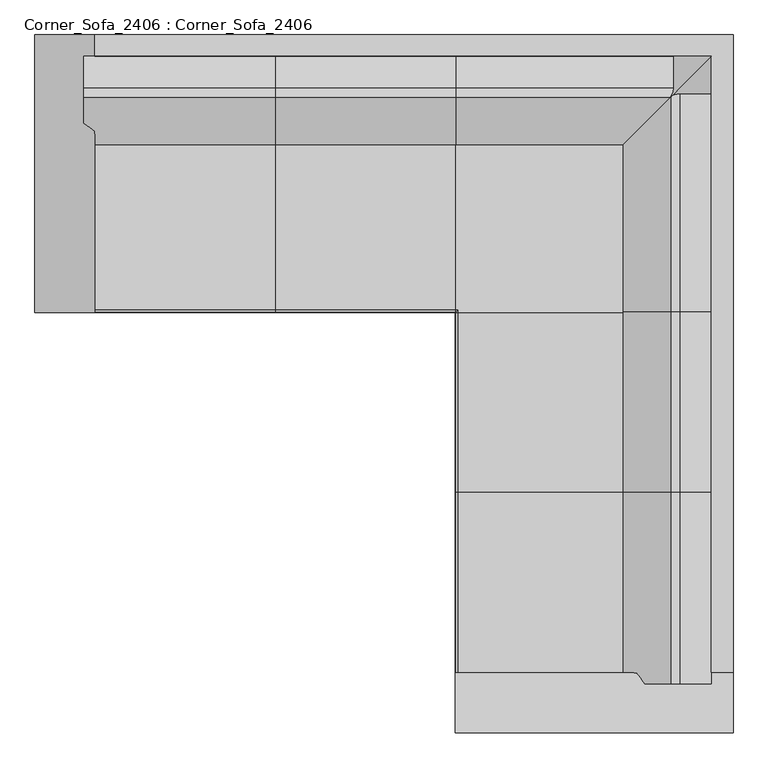
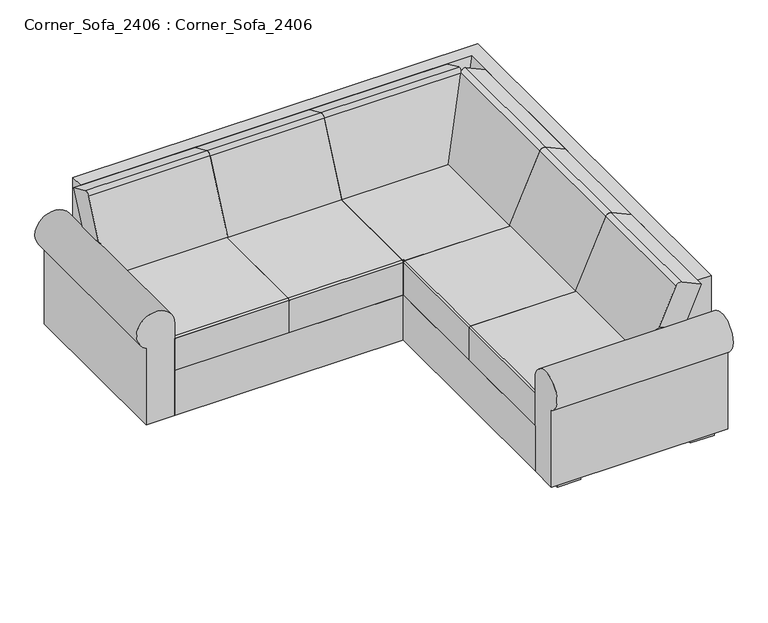
"""IFC4 building model written with IfcOpenShell, lengths in millimetres: furniture geometry, Corner_Sofa_2406 : Corner_Sofa_2406."""

from ifc_helpers import new_model, si_unit, point, frame, frame_2d, origin, origin_with_axes, place, context, project, spatial, polyline, circle_curve, ellipse_curve, trimmed, segment, composite_curve, outline, extrude, faceted_brep, source, transform, mapped, element, save
from ifc_brep_helpers import plane_surface, cylinder_surface, advanced_brep


def corner_sofa_2406_corner_sofa_2406_47bd3d46(model_context):
    return source(origin(), model_context, "Body", "SolidModel", [
        faceted_brep([(-1079.5, -939.8, 38.1), (-1079.5, -939.8, 292.1), (-1079.5, -304.8, 292.1), (-1079.5, -72.9694236, 812.8), (-1079.5, 0.0, 812.8), (-1079.5, 0.0, 38.1), (139.7, -939.8, 38.1), (139.7, -939.8, 292.1), (139.7, -2159.0, 292.1), (774.7, -2159.0, 292.1), (774.7, -304.8, 292.1), (1006.5305764, -72.9694236, 812.8), (1006.5305764, -2159.0, 812.8), (1079.5, -2159.0, 812.8), (1079.5, 0.0, 812.8), (1079.5, 0.0, 38.1), (1079.5, -2159.0, 38.1), (139.7, -2159.0, 38.1)], [[[0, 1, 2, 3, 4, 5]], [[1, 0, 6, 7]], [[2, 1, 7, 8, 9, 10]], [[3, 2, 10, 11]], [[4, 3, 11, 12, 13, 14]], [[5, 4, 14, 15]], [[0, 5, 15, 16, 17, 6]], [[9, 8, 17, 16, 13, 12]], [[7, 6, 17, 8]], [[10, 9, 12, 11]], [[14, 13, 16, 15]]]),
        advanced_brep(
        [(-1079.5, 0.0, 558.8), (-1079.5, 0.0, 38.1), (-1231.9, 0.0, 38.1), (-1231.9, 0.0, 470.811819), (-1079.5, -939.8, 558.8), (-1231.9, -939.8, 470.811819), (-1231.9, -939.8, 38.1), (-1079.5, -939.8, 38.1), (-1079.5, -939.8, 474.1924341), (-1079.5, -939.8, 483.73201)],
        [
            (0, 1),
            (1, 2),
            (2, 3),
            (3, 0, circle_curve(frame((-1181.1, 0.0, 558.8), z_axis=(0.0, 1.0, 0.0), x_axis=(1.0, 0.0, 0.0)), 101.6)),
            (4, 5, circle_curve(frame((-1181.1, -939.8, 558.8), z_axis=(0.0, -1.0, 0.0), x_axis=(1.0, 0.0, 0.0)), 101.6)),
            (5, 6),
            (6, 7),
            (7, 8),
            (8, 9),
            (9, 4),
            (0, 4),
            (7, 1),
            (6, 2),
            (5, 3),
        ],
        [
            plane_surface(frame((-1079.5, 0.0, 0.0), z_axis=(0.0, 1.0, 0.0), x_axis=(0.0, 0.0, 1.0))),
            plane_surface(frame((-1079.5, -939.8, 0.0), z_axis=(0.0, -1.0, 0.0), x_axis=(0.0, 0.0, 1.0))),
            plane_surface(frame((-1079.5, 0.0, 558.8), z_axis=(1.0, 0.0, 0.0), x_axis=(0.0, -1.0, 0.0))),
            plane_surface(frame((-1079.5, 0.0, 38.1), z_axis=(0.0, 0.0, -1.0), x_axis=(0.0, -1.0, 0.0))),
            plane_surface(frame((-1231.9, 0.0, 38.1), z_axis=(-1.0, 0.0, 0.0), x_axis=(0.0, -1.0, 0.0))),
            cylinder_surface(frame((-1181.1, 0.0, 558.8), z_axis=(0.0, 1.0, 0.0), x_axis=(1.0, 0.0, 0.0)), 101.6),
        ],
        [
            (0, [[1, 2, 3, 4]]),
            (1, [[5, 6, 7, 8, 9, 10]]),
            (2, [[-1, 11, -10, -9, -8, 12]]),
            (3, [[-2, -12, -7, 13]]),
            (4, [[-3, -13, -6, 14]]),
            (5, [[-4, -14, -5, -11]]),
        ],
    ),
        advanced_brep(
        [(1079.5, -2159.0, 558.8), (1079.5, -2311.4, 470.811819), (1079.5, -2311.4, 38.1), (1079.5, -2159.0, 38.1), (139.7, -2159.0, 38.1), (139.7, -2311.4, 38.1), (139.7, -2311.4, 470.811819), (139.7, -2159.0, 558.8), (139.7, -2159.0, 483.73201), (139.7, -2159.0, 474.1924341)],
        [
            (0, 1, circle_curve(frame((1079.5, -2260.6, 558.8), z_axis=(1.0, 0.0, 0.0), x_axis=(0.0, 1.0000000000000004, 0.0)), 101.6)),
            (1, 2),
            (2, 3),
            (3, 0),
            (4, 5),
            (5, 6),
            (6, 7, circle_curve(frame((139.7, -2260.6, 558.8), z_axis=(-1.0, 0.0, 0.0), x_axis=(0.0, 1.0000000000000004, 0.0)), 101.6)),
            (7, 8),
            (8, 9),
            (9, 4),
            (0, 7),
            (6, 1),
            (5, 2),
            (4, 3),
        ],
        [
            plane_surface(frame((1079.5, -2159.0, 0.0), z_axis=(1.0, 0.0, 0.0), x_axis=(0.0, 0.0, 1.0))),
            plane_surface(frame((139.7, -2159.0, 0.0), z_axis=(-1.0, 0.0, 0.0), x_axis=(0.0, 0.0, 1.0))),
            cylinder_surface(frame((1079.5, -2260.6, 558.8), z_axis=(1.0000000000000004, 0.0, 0.0), x_axis=(0.0, 1.0000000000000004, 0.0)), 101.6),
            plane_surface(frame((1079.5, -2311.4, 470.811819), z_axis=(0.0, -1.0, 0.0), x_axis=(-1.0, 0.0, 0.0))),
            plane_surface(frame((1079.5, -2311.4, 38.1), z_axis=(0.0, 0.0, -1.0), x_axis=(-1.0, 0.0, 0.0))),
            plane_surface(frame((1079.5, -2159.0, 38.1), z_axis=(0.0, 1.0, 0.0), x_axis=(-1.0, 0.0, 0.0))),
        ],
        [
            (0, [[1, 2, 3, 4]]),
            (1, [[5, 6, 7, 8, 9, 10]]),
            (2, [[-1, 11, -7, 12]]),
            (3, [[-2, -12, -6, 13]]),
            (4, [[-3, -13, -5, 14]]),
            (5, [[-4, -14, -10, -9, -8, -11]]),
        ],
    ),
        extrude(outline(composite_curve([segment(polyline([(-330.2, 292.1), (-939.8, 292.1), (-939.8, 474.1924341), (-939.0137794, 474.1924341)]), True, "CONTINUOUS"), segment(trimmed(circle_curve(frame_2d((-926.8744304, 470.460651)), 12.7), [point((-939.0137794, 474.1924341))], [point((-930.6062136, 482.6))], False, "CARTESIAN"), True, "CONTINUOUS"), segment(polyline([(-930.6062136, 482.6), (-330.2, 482.6), (-330.2, 292.1)]), True, "CONTINUOUS")], self_intersect=False)), frame((-1079.5, 0.0, 0.0), z_axis=(1.0, 0.0, 0.0), x_axis=(0.0, 1.0, 0.0)), (0.0, 0.0, 1.0), 609.6),
        extrude(outline(composite_curve([segment(polyline([(-330.2, 292.1), (-939.8, 292.1), (-939.8, 474.1924341), (-939.0137794, 474.1924341)]), True, "CONTINUOUS"), segment(trimmed(circle_curve(frame_2d((-926.8744304, 470.460651)), 12.7), [point((-939.0137794, 474.1924341))], [point((-930.6062136, 482.6))], False, "CARTESIAN"), True, "CONTINUOUS"), segment(polyline([(-930.6062136, 482.6), (-330.2, 482.6), (-330.2, 292.1)]), True, "CONTINUOUS")], self_intersect=False)), frame((-469.9, 0.0, 0.0), z_axis=(1.0, 0.0, 0.0), x_axis=(0.0, 1.0, 0.0)), (0.0, 0.0, 1.0), 609.6),
        advanced_brep(
        [(749.3, -939.8, 482.6), (749.3, -330.2, 482.6), (139.7, -330.2, 482.6), (139.7, -930.6062136, 482.6), (148.8937864, -930.6062136, 482.6), (148.8937864, -939.8, 482.6), (749.3, -939.8, 292.1), (139.7, -939.8, 292.1), (139.7, -330.2, 292.1), (749.3, -330.2, 292.1), (139.7, -939.8, 474.1924341), (139.7, -939.0137794, 474.1924341), (140.4862206, -939.8, 474.1924341), (140.4862206, -939.0137794, 474.1924341)],
        [
            (0, 1),
            (1, 2),
            (2, 3),
            (3, 4),
            (4, 5),
            (5, 0),
            (6, 7),
            (7, 8),
            (8, 9),
            (9, 6),
            (0, 6),
            (9, 1),
            (8, 2),
            (7, 10),
            (10, 11),
            (11, 3, circle_curve(frame((139.7, -926.8744304, 470.460651), z_axis=(-1.0, 0.0, 0.0), x_axis=(0.0, -1.0, 0.0)), 12.7)),
            (5, 12, circle_curve(frame((152.6255696, -939.8, 470.460651), z_axis=(0.0, -1.0, 0.0), x_axis=(-1.0000000000000002, 0.0, 0.0)), 12.7)),
            (12, 10),
            (13, 4, ellipse_curve(frame((152.6255696, -926.8744304, 470.460651), z_axis=(-0.7071067811865469, 0.7071067811865481, 0.0), x_axis=(0.7071067811865481, 0.7071067811865469, 0.0)), 17.9605122, 12.7)),
            (11, 13),
            (12, 13),
        ],
        [
            plane_surface(frame((749.3, -939.8, 482.6), z_axis=(0.0, 0.0, 1.0), x_axis=(0.0, 1.0, 0.0))),
            plane_surface(frame((749.3, -939.8, 292.1), z_axis=(0.0, 0.0, -1.0), x_axis=(0.0, -1.0, 0.0))),
            plane_surface(frame((749.3, -939.8, 482.6), z_axis=(1.0, 0.0, 0.0), x_axis=(0.0, 0.0, -1.0))),
            plane_surface(frame((749.3, -330.2, 482.6), z_axis=(0.0, 1.0, 0.0), x_axis=(0.0, 0.0, -1.0))),
            plane_surface(frame((139.7, -330.2, 482.6), z_axis=(-1.0, 0.0, 0.0), x_axis=(0.0, 0.0, -1.0))),
            plane_surface(frame((139.7, -939.8, 482.6), z_axis=(0.0, -1.0, 0.0), x_axis=(0.0, 0.0, -1.0))),
            cylinder_surface(frame((-1079.5, -926.8744304, 470.460651), z_axis=(1.0, 0.0, 0.0), x_axis=(0.0, -1.0, 0.0)), 12.7),
            plane_surface(frame((-1079.5, -939.0137794, 474.1924341), z_axis=(0.0, 0.0, 1.0), x_axis=(1.0, 0.0, 0.0))),
            cylinder_surface(frame((152.6255696, -939.8, 470.460651), z_axis=(0.0, -1.0000000000000004, 0.0), x_axis=(-1.0000000000000002, 0.0, 0.0)), 12.7),
        ],
        [
            (0, [[1, 2, 3, 4, 5, 6]]),
            (1, [[7, 8, 9, 10]]),
            (2, [[-1, 11, -10, 12]]),
            (3, [[-2, -12, -9, 13]]),
            (4, [[-8, 14, 15, 16, -3, -13]]),
            (5, [[-7, -11, -6, 17, 18, -14]]),
            (6, [[19, -4, -16, 20]]),
            (7, [[21, -20, -15, -18]]),
            (8, [[-19, -21, -17, -5]]),
        ],
    ),
        extrude(outline(composite_curve([segment(polyline([(292.1, 139.7), (292.1, 749.3), (482.6, 749.3), (482.6, 148.8937864)]), True, "CONTINUOUS"), segment(trimmed(circle_curve(frame_2d((470.460651, 152.6255696)), 12.7), [point((482.6, 148.8937864))], [point((474.1924341, 140.4862206))], False, "CARTESIAN"), True, "CONTINUOUS"), segment(polyline([(474.1924341, 140.4862206), (474.1924341, 139.7), (292.1, 139.7)]), True, "CONTINUOUS")], self_intersect=False)), frame((0.0, -2159.0, 0.0), z_axis=(0.0, 1.0, 0.0), x_axis=(0.0, 0.0, 1.0)), (0.0, 0.0, 1.0), 609.6),
        extrude(outline(composite_curve([segment(polyline([(292.1, 139.7), (292.1, 749.3), (482.6, 749.3), (482.6, 148.8937864)]), True, "CONTINUOUS"), segment(trimmed(circle_curve(frame_2d((470.460651, 152.6255696)), 12.7), [point((482.6, 148.8937864))], [point((474.1924341, 140.4862206))], False, "CARTESIAN"), True, "CONTINUOUS"), segment(polyline([(474.1924341, 140.4862206), (474.1924341, 139.7), (292.1, 139.7)]), True, "CONTINUOUS")], self_intersect=False)), frame((0.0, -1549.4, 0.0), z_axis=(0.0, 1.0, 0.0), x_axis=(0.0, 0.0, 1.0)), (0.0, 0.0, 1.0), 609.6),
        advanced_brep(
        [(-1116.8137794, -298.9707144, 648.6582788), (-1079.5, -325.2578441, 589.6164189), (-1079.5, -371.2884895, 486.2298964), (-469.1137794, -371.2884895, 486.2298964), (-469.1137794, -210.9228347, 846.4170544), (-469.1137794, -210.0920381, 848.2830543), (-1116.8137794, -210.0920381, 848.2830543), (-1116.8137794, -210.9228347, 846.4170544), (-469.1137794, -72.9694236, 812.8), (-469.1137794, -243.6661891, 429.4087874), (-1079.5, -243.6661891, 429.4087874), (-1079.5, -197.6355436, 532.7953098), (-1116.8137794, -171.348414, 591.8371697), (-1116.8137794, -72.9694236, 812.8), (-1116.8137794, -177.3876694, 859.2899983), (-1116.8137794, -179.2536692, 860.120795), (-469.1137794, -179.2536692, 860.120795), (-469.1137794, -177.3876694, 859.2899983)],
        [
            (0, 1),
            (1, 2),
            (2, 3),
            (3, 4),
            (4, 5),
            (5, 6),
            (6, 7),
            (7, 0),
            (8, 9),
            (9, 10),
            (10, 11),
            (11, 12),
            (12, 13),
            (13, 8),
            (13, 14),
            (14, 15),
            (15, 16),
            (16, 17),
            (17, 8),
            (12, 0),
            (6, 15, circle_curve(frame((-1116.8137794, -188.2363817, 837.4343419), z_axis=(-1.0, 0.0, 0.0), x_axis=(0.0, -1.0, 0.0)), 24.4000876)),
            (11, 1),
            (10, 2),
            (9, 3),
            (16, 5, circle_curve(frame((-469.1137794, -188.2363817, 837.4343419), z_axis=(1.0, 0.0, 0.0), x_axis=(0.0, -1.0, 0.0)), 24.4000876)),
        ],
        [
            plane_surface(frame((-469.1137794, -200.591724, 869.621109), z_axis=(0.0, -0.9135454576426002, 0.40673664307580193), x_axis=(-1.0, 0.0, 0.0))),
            plane_surface(frame((-469.1137794, -72.9694236, 812.8), z_axis=(0.0, 0.9135454576426002, -0.40673664307580193), x_axis=(1.0, 0.0, 0.0))),
            plane_surface(frame((-469.1137794, -200.591724, 869.621109), z_axis=(0.0, 0.4067366430758019, 0.9135454576426002), x_axis=(0.0, 0.9135454576426002, -0.4067366430758019))),
            plane_surface(frame((-1116.8137794, -200.591724, 869.621109), z_axis=(-1.0, 0.0, 0.0), x_axis=(0.0, 0.9135454576425998, -0.4067366430758028))),
            plane_surface(frame((-1116.8137794, -298.9707144, 648.6582788), z_axis=(-0.8660254037844393, -0.20336832153790044, -0.4567727288212995), x_axis=(0.0, 0.9135454576426004, -0.4067366430758015))),
            plane_surface(frame((-1079.5, -325.2578441, 589.6164189), z_axis=(-1.0, 0.0, 0.0), x_axis=(0.0, 0.9135454576426002, -0.4067366430758019))),
            plane_surface(frame((-1079.5, -371.2884895, 486.2298964), z_axis=(0.0, -0.40673664307580226, -0.9135454576426), x_axis=(0.0, 0.9135454576426, -0.40673664307580226))),
            plane_surface(frame((-469.1137794, -371.2884895, 486.2298964), z_axis=(1.0, 0.0, 0.0), x_axis=(0.0, 0.9135454576426002, -0.4067366430758019))),
            cylinder_surface(frame((-1116.8137794, -188.2363817, 837.4343419), z_axis=(1.0, 0.0, 0.0), x_axis=(0.0, -1.0, 0.0)), 24.4000876),
        ],
        [
            (0, [[1, 2, 3, 4, 5, 6, 7, 8]]),
            (1, [[9, 10, 11, 12, 13, 14]]),
            (2, [[-14, 15, 16, 17, 18, 19]]),
            (3, [[-13, 20, -8, -7, 21, -16, -15]]),
            (4, [[-1, -20, -12, 22]]),
            (5, [[-2, -22, -11, 23]]),
            (6, [[-3, -23, -10, 24]]),
            (7, [[-9, -19, -18, 25, -5, -4, -24]]),
            (8, [[-6, -25, -17, -21]]),
        ],
    ),
        advanced_brep(
        [(-469.9, -371.2884895, 486.2298964), (140.4862206, -371.2884895, 486.2298964), (140.4862206, -210.9228347, 846.4170544), (140.4862206, -210.0920381, 848.2830543), (-469.9, -210.0920381, 848.2830543), (-469.9, -210.9228347, 846.4170544), (140.4862206, -72.9694236, 812.8), (140.4862206, -243.6661891, 429.4087874), (-469.9, -243.6661891, 429.4087874), (-469.9, -72.9694236, 812.8), (-469.9, -177.3876694, 859.2899983), (-469.9, -179.2536692, 860.120795), (140.4862206, -179.2536692, 860.120795), (140.4862206, -177.3876694, 859.2899983)],
        [
            (0, 1),
            (1, 2),
            (2, 3),
            (3, 4),
            (4, 5),
            (5, 0),
            (6, 7),
            (7, 8),
            (8, 9),
            (9, 6),
            (9, 10),
            (10, 11),
            (11, 12),
            (12, 13),
            (13, 6),
            (8, 0),
            (4, 11, circle_curve(frame((-469.9, -188.2363817, 837.4343419), z_axis=(-1.0, 0.0, 0.0), x_axis=(0.0, -1.0, 0.0)), 24.4000876)),
            (7, 1),
            (12, 3, circle_curve(frame((140.4862206, -188.2363817, 837.4343419), z_axis=(1.0, 0.0, 0.0), x_axis=(0.0, -1.0, 0.0)), 24.4000876)),
        ],
        [
            plane_surface(frame((140.4862206, -200.591724, 869.621109), z_axis=(0.0, -0.9135454576426002, 0.40673664307580193), x_axis=(-1.0, 0.0, 0.0))),
            plane_surface(frame((140.4862206, -72.9694236, 812.8), z_axis=(0.0, 0.9135454576426002, -0.40673664307580193), x_axis=(1.0, 0.0, 0.0))),
            plane_surface(frame((140.4862206, -200.591724, 869.621109), z_axis=(0.0, 0.4067366430758019, 0.9135454576426003), x_axis=(0.0, 0.9135454576426003, -0.4067366430758019))),
            plane_surface(frame((-469.9, -200.591724, 869.621109), z_axis=(-1.0000000000000002, 0.0, 0.0), x_axis=(0.0, 0.9135454576426003, -0.4067366430758019))),
            plane_surface(frame((-469.9, -371.2884895, 486.2298964), z_axis=(0.0, -0.406736643075802, -0.9135454576426002), x_axis=(0.0, 0.9135454576426002, -0.406736643075802))),
            plane_surface(frame((140.4862206, -371.2884895, 486.2298964), z_axis=(1.0000000000000002, 0.0, 0.0), x_axis=(0.0, 0.9135454576426003, -0.4067366430758019))),
            cylinder_surface(frame((-1116.8137794, -188.2363817, 837.4343419), z_axis=(1.0, 0.0, 0.0), x_axis=(0.0, -1.0, 0.0)), 24.4000876),
        ],
        [
            (0, [[1, 2, 3, 4, 5, 6]]),
            (1, [[7, 8, 9, 10]]),
            (2, [[-10, 11, 12, 13, 14, 15]]),
            (3, [[-9, 16, -6, -5, 17, -12, -11]]),
            (4, [[-1, -16, -8, 18]]),
            (5, [[-7, -15, -14, 19, -3, -2, -18]]),
            (6, [[-4, -19, -13, -17]]),
        ],
    ),
        advanced_brep(
        [(139.7, -371.2884895, 486.2298964), (706.2350262, -371.2884895, 486.2298964), (866.600681, -210.9228347, 846.4170544), (867.4314777, -210.0920381, 848.2830543), (139.7, -210.0920381, 848.2830543), (139.7, -210.9228347, 846.4170544), (139.7, -72.9694236, 812.8), (876.9317918, -72.9694236, 812.8), (706.2350262, -243.6661891, 429.4087874), (139.7, -243.6661891, 429.4087874), (139.7, -179.2536692, 860.120795), (139.7, -177.3876694, 859.2899983), (876.9317918, -177.3876694, 859.2899983), (876.9317918, -179.2536692, 860.120795)],
        [
            (0, 1),
            (1, 2),
            (2, 3),
            (3, 4),
            (4, 5),
            (5, 0),
            (6, 7),
            (7, 8),
            (8, 9),
            (9, 6),
            (9, 0),
            (4, 10, circle_curve(frame((139.7, -188.2363817, 837.4343419), z_axis=(-1.0, 0.0, 0.0), x_axis=(0.0, -1.0, 0.0)), 24.4000876)),
            (10, 11),
            (11, 6),
            (8, 1),
            (7, 12),
            (12, 13),
            (13, 3, ellipse_curve(frame((867.0160793, -188.2363817, 837.4343419), z_axis=(0.926309308298545, -0.15324369958044406, -0.3441909846268057), x_axis=(0.37676393850721845, 0.37676393850721107, 0.8462256609681977)), 26.341188, 24.4000876)),
            (10, 13),
        ],
        [
            plane_surface(frame((139.7, -325.2578441, 589.6164189), z_axis=(0.0, -0.9135454576426002, 0.406736643075802), x_axis=(0.0, -0.406736643075802, -0.9135454576426002))),
            plane_surface(frame((139.7, -197.6355436, 532.7953098), z_axis=(0.0, 0.9135454576426002, -0.406736643075802), x_axis=(0.0, 0.406736643075802, 0.9135454576426002))),
            plane_surface(frame((139.7, -200.591724, 869.621109), z_axis=(-1.0, 0.0, 0.0), x_axis=(0.0, 0.9135454576425998, -0.40673664307580293))),
            plane_surface(frame((139.7, -371.2884895, 486.2298964), z_axis=(0.0, -0.406736643075802, -0.9135454576426002), x_axis=(0.0, 0.9135454576426002, -0.406736643075802))),
            plane_surface(frame((706.2350262, -371.2884895, 486.2298964), z_axis=(0.926309308298545, -0.15324369958044406, -0.3441909846268057), x_axis=(0.0, 0.9135454576426002, -0.406736643075802))),
            plane_surface(frame((876.9317918, -200.591724, 869.621109), z_axis=(0.0, 0.40673664307580276, 0.9135454576425999), x_axis=(0.0, 0.9135454576425999, -0.40673664307580276))),
            cylinder_surface(frame((-1116.8137794, -188.2363817, 837.4343419), z_axis=(1.0, 0.0, 0.0), x_axis=(0.0, -1.0, 0.0)), 24.4000876),
        ],
        [
            (0, [[1, 2, 3, 4, 5, 6]]),
            (1, [[7, 8, 9, 10]]),
            (2, [[-10, 11, -6, -5, 12, 13, 14]]),
            (3, [[-1, -11, -9, 15]]),
            (4, [[-8, 16, 17, 18, -3, -2, -15]]),
            (5, [[-7, -14, -13, 19, -17, -16]]),
            (6, [[-4, -18, -19, -12]]),
        ],
    ),
        advanced_brep(
        [(708.2115105, -1548.6137794, 486.2298964), (708.2115105, -2159.0, 486.2298964), (754.2421559, -2159.0, 589.6164189), (780.5292856, -2196.3137794, 648.6582788), (868.5771653, -2196.3137794, 846.4170544), (869.4079619, -2196.3137794, 848.2830543), (869.4079619, -1548.6137794, 848.2830543), (868.5771653, -1548.6137794, 846.4170544), (1006.5305764, -1548.6137794, 812.8), (1006.5305764, -2196.3137794, 812.8), (908.151586, -2196.3137794, 591.8371697), (881.8644564, -2159.0, 532.7953098), (835.8338109, -2159.0, 429.4087874), (835.8338109, -1548.6137794, 429.4087874), (900.2463308, -1548.6137794, 860.120795), (902.1123306, -1548.6137794, 859.2899983), (902.1123306, -2196.3137794, 859.2899983), (900.2463308, -2196.3137794, 860.120795)],
        [
            (0, 1),
            (1, 2),
            (2, 3),
            (3, 4),
            (4, 5),
            (5, 6),
            (6, 7),
            (7, 0),
            (8, 9),
            (9, 10),
            (10, 11),
            (11, 12),
            (12, 13),
            (13, 8),
            (13, 0),
            (6, 14, circle_curve(frame((891.2636183, -1548.6137794, 837.4343419), z_axis=(0.0, 1.0, 0.0), x_axis=(-0.9999999999999999, 0.0, 0.0)), 24.4000876)),
            (14, 15),
            (15, 8),
            (12, 1),
            (11, 2),
            (10, 3),
            (9, 16),
            (16, 17),
            (17, 5, circle_curve(frame((891.2636183, -2196.3137794, 837.4343419), z_axis=(0.0, -1.0, 0.0), x_axis=(-0.9999999999999999, 0.0, 0.0)), 24.4000876)),
            (14, 17),
        ],
        [
            plane_surface(frame((708.2115105, -1548.6137794, 486.2298964), z_axis=(-0.9135454576426002, 0.0, 0.40673664307580193), x_axis=(-0.40673664307580193, 0.0, -0.9135454576426002))),
            plane_surface(frame((835.8338109, -1548.6137794, 429.4087874), z_axis=(0.9135454576426002, 0.0, -0.40673664307580193), x_axis=(0.40673664307580193, 0.0, 0.9135454576426002))),
            plane_surface(frame((878.908276, -1548.6137794, 869.621109), z_axis=(0.0, 1.0000000000000002, 0.0), x_axis=(0.9135454576426003, 0.0, -0.4067366430758019))),
            plane_surface(frame((708.2115105, -1548.6137794, 486.2298964), z_axis=(-0.4067366430758019, 0.0, -0.9135454576426003), x_axis=(0.9135454576426003, 0.0, -0.4067366430758019))),
            plane_surface(frame((708.2115105, -2159.0, 486.2298964), z_axis=(0.0, -1.0000000000000002, 0.0), x_axis=(0.9135454576426003, 0.0, -0.4067366430758019))),
            plane_surface(frame((754.2421559, -2159.0, 589.6164189), z_axis=(-0.20336832153790022, -0.8660254037844399, -0.45677272882129855), x_axis=(0.9135454576426003, 0.0, -0.4067366430758019))),
            plane_surface(frame((780.5292856, -2196.3137794, 648.6582788), z_axis=(0.0, -1.0000000000000002, 0.0), x_axis=(0.9135454576426003, 0.0, -0.4067366430758019))),
            plane_surface(frame((878.908276, -2196.3137794, 869.621109), z_axis=(0.4067366430758019, 0.0, 0.9135454576426003), x_axis=(0.9135454576426003, 0.0, -0.4067366430758019))),
            cylinder_surface(frame((891.2636183, -200.591724, 837.4343419), z_axis=(0.0, -0.9999999999999998, 0.0), x_axis=(-0.9999999999999999, 0.0, 0.0)), 24.4000876),
        ],
        [
            (0, [[1, 2, 3, 4, 5, 6, 7, 8]]),
            (1, [[9, 10, 11, 12, 13, 14]]),
            (2, [[-14, 15, -8, -7, 16, 17, 18]]),
            (3, [[-1, -15, -13, 19]]),
            (4, [[-2, -19, -12, 20]]),
            (5, [[-3, -20, -11, 21]]),
            (6, [[-10, 22, 23, 24, -5, -4, -21]]),
            (7, [[-9, -18, -17, 25, -23, -22]]),
            (8, [[-6, -24, -25, -16]]),
        ],
    ),
        advanced_brep(
        [(708.2115105, -939.0137794, 486.2298964), (708.2115105, -1549.4, 486.2298964), (868.5771653, -1549.4, 846.4170544), (869.4079619, -1549.4, 848.2830543), (869.4079619, -939.0137794, 848.2830543), (868.5771653, -939.0137794, 846.4170544), (1006.5305764, -939.0137794, 812.8), (1006.5305764, -1549.4, 812.8), (835.8338109, -1549.4, 429.4087874), (835.8338109, -939.0137794, 429.4087874), (900.2463308, -939.0137794, 860.120795), (902.1123306, -939.0137794, 859.2899983), (902.1123306, -1549.4, 859.2899983), (900.2463308, -1549.4, 860.120795)],
        [
            (0, 1),
            (1, 2),
            (2, 3),
            (3, 4),
            (4, 5),
            (5, 0),
            (6, 7),
            (7, 8),
            (8, 9),
            (9, 6),
            (9, 0),
            (4, 10, circle_curve(frame((891.2636183, -939.0137794, 837.4343419), z_axis=(0.0, 1.0, 0.0), x_axis=(-0.9999999999999999, 0.0, 0.0)), 24.4000876)),
            (10, 11),
            (11, 6),
            (8, 1),
            (7, 12),
            (12, 13),
            (13, 3, circle_curve(frame((891.2636183, -1549.4, 837.4343419), z_axis=(0.0, -1.0, 0.0), x_axis=(-0.9999999999999999, 0.0, 0.0)), 24.4000876)),
            (10, 13),
        ],
        [
            plane_surface(frame((708.2115105, -939.0137794, 486.2298964), z_axis=(-0.9135454576426002, 0.0, 0.40673664307580193), x_axis=(-0.40673664307580193, 0.0, -0.9135454576426002))),
            plane_surface(frame((835.8338109, -939.0137794, 429.4087874), z_axis=(0.9135454576426002, 0.0, -0.40673664307580193), x_axis=(0.40673664307580193, 0.0, 0.9135454576426002))),
            plane_surface(frame((878.908276, -939.0137794, 869.621109), z_axis=(0.0, 1.0000000000000002, 0.0), x_axis=(0.9135454576426003, 0.0, -0.4067366430758019))),
            plane_surface(frame((708.2115105, -939.0137794, 486.2298964), z_axis=(-0.4067366430758019, 0.0, -0.9135454576426003), x_axis=(0.9135454576426003, 0.0, -0.4067366430758019))),
            plane_surface(frame((708.2115105, -1549.4, 486.2298964), z_axis=(0.0, -1.0000000000000002, 0.0), x_axis=(0.9135454576426003, 0.0, -0.4067366430758019))),
            plane_surface(frame((878.908276, -1549.4, 869.621109), z_axis=(0.4067366430758011, 0.0, 0.9135454576426005), x_axis=(0.9135454576426005, 0.0, -0.4067366430758011))),
            cylinder_surface(frame((891.2636183, -200.591724, 837.4343419), z_axis=(0.0, -0.9999999999999998, 0.0), x_axis=(-0.9999999999999999, 0.0, 0.0)), 24.4000876),
        ],
        [
            (0, [[1, 2, 3, 4, 5, 6]]),
            (1, [[7, 8, 9, 10]]),
            (2, [[-10, 11, -6, -5, 12, 13, 14]]),
            (3, [[-1, -11, -9, 15]]),
            (4, [[-8, 16, 17, 18, -3, -2, -15]]),
            (5, [[-7, -14, -13, 19, -17, -16]]),
            (6, [[-4, -18, -19, -12]]),
        ],
    ),
        advanced_brep(
        [(708.2115105, -370.9615105, 486.2298964), (708.2115105, -939.8, 486.2298964), (868.5771653, -939.8, 846.4170544), (869.4079619, -939.8, 848.2830543), (869.4079619, -210.0920381, 848.2830543), (870.5407312, -208.6322897, 850.8272957), (1006.5305764, -939.8, 812.8), (835.8338109, -939.8, 429.4087874), (835.8338109, -370.9615105, 429.4087874), (1006.5305764, -200.2647449, 812.8), (902.1123306, -200.2647449, 859.2899983), (900.2463308, -200.2647449, 860.120795), (900.2463308, -939.8, 860.120795), (902.1123306, -939.8, 859.2899983), (871.062652, -208.437348, 851.1195615)],
        [
            (0, 1),
            (1, 2),
            (2, 3),
            (3, 4),
            (4, 5, ellipse_curve(frame((864.577804, -188.2363817, 837.4343419), z_axis=(-0.9135454576426002, 0.0, 0.40673664307580193), x_axis=(0.40673664307580176, 0.0, 0.9135454576426003)), 26.7092211, 24.4000876)),
            (5, 0),
            (6, 7),
            (7, 8),
            (8, 9),
            (9, 6),
            (9, 10),
            (10, 11),
            (11, 12),
            (12, 13),
            (13, 6),
            (8, 0),
            (5, 14, ellipse_curve(frame((1023.9085595, -188.2363817, 837.4343419), z_axis=(-0.15324369958044412, 0.926309308298545, -0.34419098462680536), x_axis=(0.9881884276487448, 0.14364777140451176, -0.053375549005312696)), 159.2240834, 24.4000876)),
            (14, 11, ellipse_curve(frame((891.2636183, -210.1804573, 837.4343419), z_axis=(-0.15324369958044412, 0.926309308298545, -0.34419098462680536), x_axis=(-0.37676393850722284, -0.3767639385072186, -0.8462256609681926)), 26.341188, 24.4000876)),
            (7, 1),
            (12, 3, circle_curve(frame((891.2636183, -939.8, 837.4343419), z_axis=(0.0, -1.0, 0.0), x_axis=(-0.9999999999999999, 0.0, 0.0)), 24.4000876)),
            (4, 14, ellipse_curve(frame((891.2636183, -188.2363817, 837.4343419), z_axis=(-0.7071067811865457, 0.7071067811865493, 0.0), x_axis=(0.7071067811865492, 0.7071067811865458, 0.0)), 34.5069348, 24.4000876)),
        ],
        [
            plane_surface(frame((878.908276, -329.4137794, 869.621109), z_axis=(-0.9135454576426002, 0.0, 0.40673664307580193), x_axis=(0.0, 1.0, 0.0))),
            plane_surface(frame((1006.5305764, -329.4137794, 812.8), z_axis=(0.9135454576426002, 0.0, -0.40673664307580193), x_axis=(0.0, -1.0, 0.0))),
            plane_surface(frame((878.908276, -939.8, 869.621109), z_axis=(0.4067366430758019, 0.0, 0.9135454576426003), x_axis=(0.9135454576426003, 0.0, -0.4067366430758019))),
            plane_surface(frame((878.908276, -200.2647449, 869.621109), z_axis=(-0.15324369958044415, 0.9263093082985452, -0.3441909846268054), x_axis=(0.9135454576426003, 0.0, -0.4067366430758019))),
            plane_surface(frame((708.2115105, -370.9615105, 486.2298964), z_axis=(-0.4067366430758019, 0.0, -0.9135454576426003), x_axis=(0.9135454576426003, 0.0, -0.4067366430758019))),
            plane_surface(frame((708.2115105, -939.8, 486.2298964), z_axis=(0.0, -1.0000000000000002, 0.0), x_axis=(0.9135454576426003, 0.0, -0.4067366430758019))),
            cylinder_surface(frame((-1116.8137794, -188.2363817, 837.4343419), z_axis=(1.0, 0.0, 0.0), x_axis=(0.0, -1.0, 0.0)), 24.4000876),
            cylinder_surface(frame((891.2636183, -200.591724, 837.4343419), z_axis=(0.0, -0.9999999999999998, 0.0), x_axis=(-0.9999999999999999, 0.0, 0.0)), 24.4000876),
        ],
        [
            (0, [[1, 2, 3, 4, 5, 6]]),
            (1, [[7, 8, 9, 10]]),
            (2, [[-10, 11, 12, 13, 14, 15]]),
            (3, [[-9, 16, -6, 17, 18, -12, -11]]),
            (4, [[-1, -16, -8, 19]]),
            (5, [[-7, -15, -14, 20, -3, -2, -19]]),
            (6, [[21, -17, -5]]),
            (7, [[-21, -4, -20, -13, -18]]),
        ],
    ),
        extrude(outline(polyline([(-1068.5682719, -892.1095227), (-1195.5682719, -892.1095227), (-1195.5682719, -765.1095227), (-1068.5682719, -765.1095227), (-1068.5682719, -892.1095227)])), origin_with_axes(), (0.0, 0.0, 1.0), 50.8),
        extrude(outline(polyline([(-1068.5682719, -180.9095227), (-1195.5682719, -180.9095227), (-1195.5682719, -53.9095227), (-1068.5682719, -53.9095227), (-1068.5682719, -180.9095227)])), origin_with_axes(), (0.0, 0.0, 1.0), 50.8),
        extrude(outline(polyline([(900.5669616, -892.1095227), (900.5669616, -765.1095227), (1027.5669616, -765.1095227), (1027.5669616, -892.1095227), (900.5669616, -892.1095227)])), origin_with_axes(), (0.0, 0.0, 1.0), 50.8),
        extrude(outline(polyline([(900.5669616, -180.9095227), (900.5669616, -53.9095227), (1027.5669616, -53.9095227), (1027.5669616, -180.9095227), (900.5669616, -180.9095227)])), origin_with_axes(), (0.0, 0.0, 1.0), 50.8),
        extrude(outline(polyline([(189.3669616, -2150.0447561), (316.3669616, -2150.0447561), (316.3669616, -2277.0447561), (189.3669616, -2277.0447561), (189.3669616, -2150.0447561)])), origin_with_axes(), (0.0, 0.0, 1.0), 50.8),
        extrude(outline(polyline([(900.5669616, -2150.0447561), (1027.5669616, -2150.0447561), (1027.5669616, -2277.0447561), (900.5669616, -2277.0447561), (900.5669616, -2150.0447561)])), origin_with_axes(), (0.0, 0.0, 1.0), 50.8),
        extrude(outline(polyline([(189.3669616, -981.6447561), (316.3669616, -981.6447561), (316.3669616, -1108.6447561), (189.3669616, -1108.6447561), (189.3669616, -981.6447561)])), origin_with_axes(), (0.0, 0.0, 1.0), 50.8),
        extrude(outline(polyline([(900.5669616, -981.6447561), (1027.5669616, -981.6447561), (1027.5669616, -1108.6447561), (900.5669616, -1108.6447561), (900.5669616, -981.6447561)])), origin_with_axes(), (0.0, 0.0, 1.0), 50.8),
    ])


if __name__ == "__main__":
    model = new_model("IFC4")
    model_context = context("Model", 3, world=origin())
    ifc_project = project(units=[si_unit("LENGTHUNIT", "METRE", prefix="MILLI")], contexts=[model_context])
    site = spatial("IfcSite", under=ifc_project)
    building = spatial("IfcBuilding", under=site)
    placement = place(None, origin())
    corner_sofa_2406_corner_sofa_2406_shape = corner_sofa_2406_corner_sofa_2406_47bd3d46(model_context)
    element("IfcFurniture", 1, ObjectType="Corner_Sofa_2406 : Corner_Sofa_2406", at=placement, inside=building, context=model_context, shape_type="MappedRepresentation", body=[
        mapped(corner_sofa_2406_corner_sofa_2406_shape, transform((0.0, 0.0, 0.0), x_axis=(1.0, 0.0, 0.0), y_axis=(0.0, 1.0, 0.0), z_axis=(0.0, 0.0, 1.0))),
    ])
    save(model, "model.ifc")

# Revit data of these elements
# Type "Corner_Sofa_2406 : Corner_Sofa_2406"
#   Fabric = none
#   Default Elevation = 0
# Element 1 (IfcFurniture, "Corner_Sofa_2406 : Corner_Sofa_2406")
#   Materials on its faces: "Default Wall"
# Materials
#   "Default Wall": colour RGB 128 128 128, transparency 0, Cost = 0
